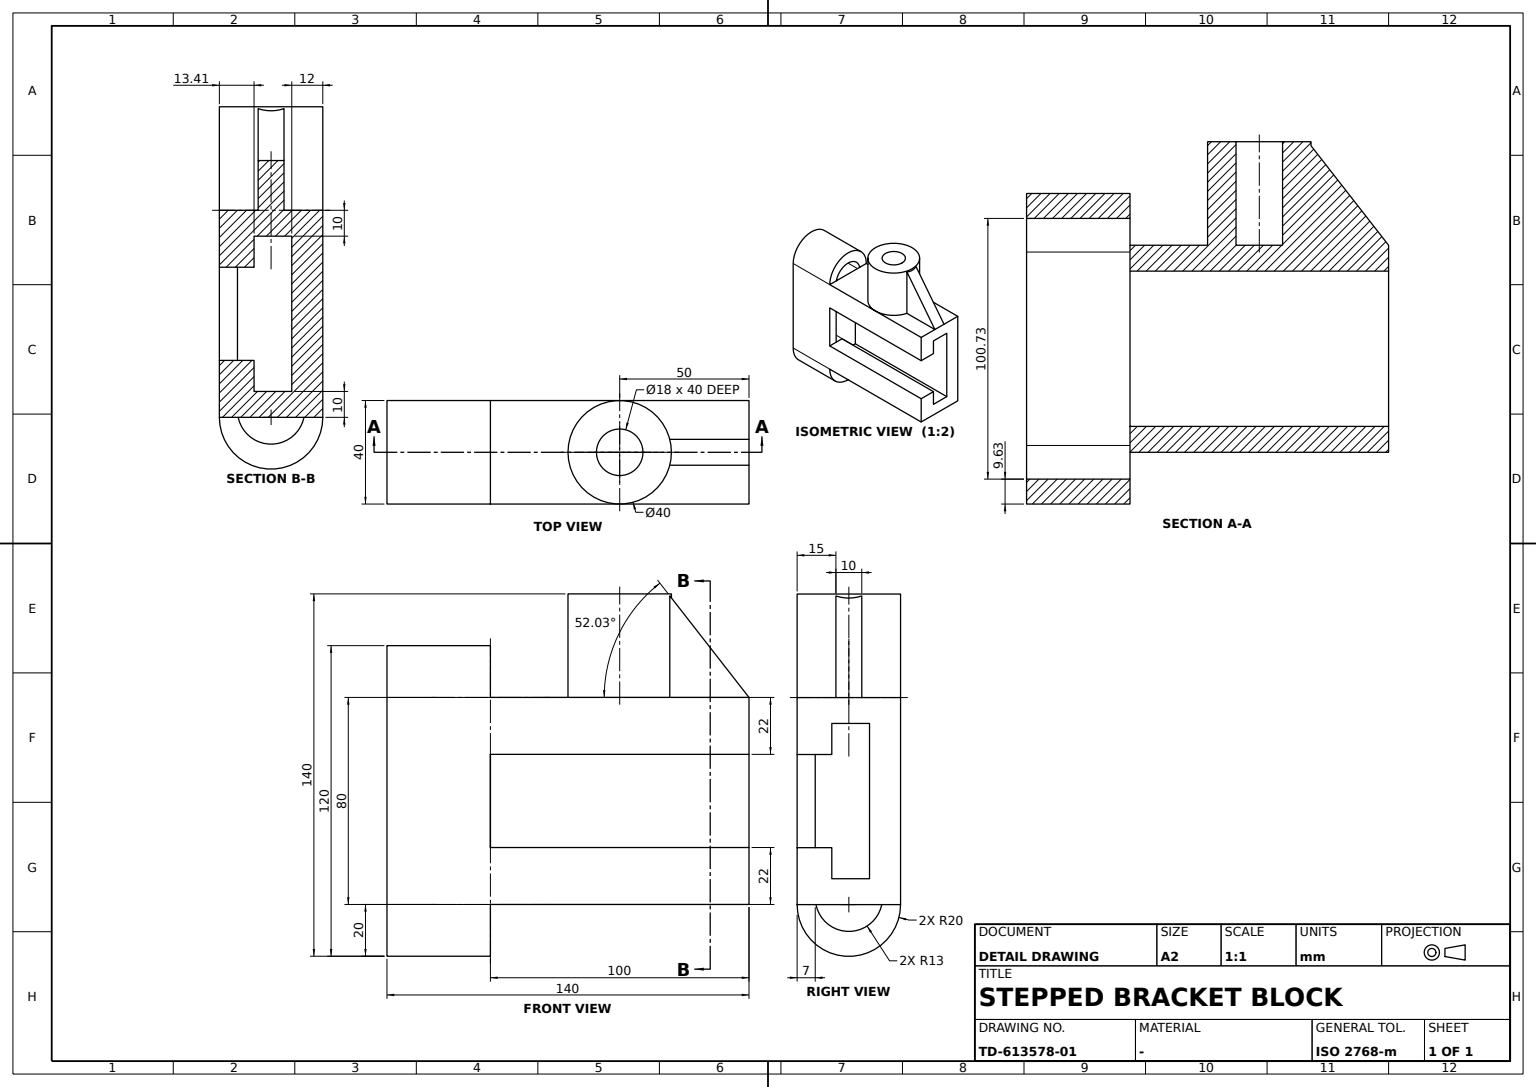
CATIA V5 part; units mm, degrees
sketch "Sketch1" plane through (0, 0, 0) normal (1, 0, 0) x (0, 1, 0)
  point P0 (-20, 40)
  line L0 (-20, 40) -> (20, 40)
  line L1 (20, 40) -> (20, -40)
  point P1 (20, -40)
  line L2 (20, -40) -> (-20, -40)
  point P2 (-20, -40)
  line L3 (-20, -40) -> (-20, -18)
  line L4 (-20, -18) -> (-6.5877, -18)
  line L5 (-6.5877, -18) -> (-6.5877, -30)
  line L6 (-6.5877, -30) -> (8, -30)
  line L7 (8, -30) -> (8, 30)
  line L8 (8, 30) -> (-6.5877, 30)
  point P3 (-6.5877, 30)
  line L9 (-6.5877, 30) -> (-6.5877, 18)
  line L10 (-6.5877, 18) -> (-20, 18)
  point P4 (-20, 18)
  line L11 (-20, 18) -> (-20, 40)
  point P5 (-20, 40)
  dimension "length L2" = 40
  dimension "distance L7 L1" = 12
  dimension "length L1" = 80
  dimension "length L3" = 22
  dimension "length L5" = 12
  dimension "length L11" = 22
  dimension "length L9" = 12
  constraint horizontal L0 x-axis
  constraint horizontal L2 x-axis
  constraint horizontal L4 x-axis
  constraint horizontal L6 x-axis
  constraint horizontal L8 x-axis
  constraint horizontal L10 x-axis
  constraint vertical L1 y-axis
  constraint vertical L3 y-axis
  constraint vertical L5 y-axis
  constraint vertical L7 y-axis
  constraint vertical L9 y-axis
  constraint vertical L11 y-axis
  constraint coincidence P3 L5
  constraint coincidence P4 L3
  constraint coincidence P5 L0
  constraint coincidence P5 P0
  constraint symmetry P2 P1 y-axis
  constraint symmetry L0 L2 x-axis
extrude "Pad1" add sketch "Sketch1" against normal blind 100
sketch "Sketch2" plane through (0, 0, 40) normal (0, 0, 1) x (1, 0, 0)
  circle A0 centre (-50, 0) radius 9
  point P0 (-50, 0)
  circle A1 centre (-50, 0) radius 20
  dimension "distance y axis P0" = 50
  dimension "radius A0" = 9
  dimension "radius A1" = 20
  constraint coincidence P0 x-axis
extrude "Pad2" add sketch "Sketch2" along normal blind 40
ref_plane "Plane1" through (-50, 0, 0) normal (1, 0, 0) x (0, 1, 0)
sketch "Sketch3" plane through (0, 0, 0) normal (0, 1, 0) x (-1, 0, 0)
  point P0 (0, 40)
  line L0 (0, 40) -> (31.2151, 40)
  point P1 (31.2151, 40)
  line L1 (31.2151, 40) -> (31.2151, 80)
  point P2 (31.2151, 80)
  line L2 (31.2151, 80) -> (0, 40)
  line L3 (30, 80) -> (70, 80) construction
  line L4 (0, 40) -> (100, 40) construction
  constraint coincidence P0 y-axis
  constraint coincidence P2 L3
  constraint coincidence P1 L4
  constraint horizontal L0 x-axis
  constraint vertical L1 y-axis
extrude "Pad3" add sketch "Sketch3" along normal mid plane 10
sketch "Sketch4" plane through (-100, 0, 0) normal (-1, 0, 0) x (0, -1, 0)
  line L0 (-20, 40) -> (20, 40)
  line L1 (20, 40) -> (20, -40)
  line L2 (20, -40) -> (-20, -40)
  line L3 (-20, -40) -> (-20, 40)
  line L4 (-20, 40) -> (20, 40) construction
  line L5 (20, 40) -> (20, 18) construction
  line L6 (-20, -40) -> (-20, 40) construction
  line L7 (20, -40) -> (-20, -40) construction
  constraint horizontal L0 x-axis
  constraint horizontal L2 x-axis
  constraint vertical L1 y-axis
  constraint vertical L3 y-axis
  constraint coincidence L4 L0
  constraint coincidence L1 L5
  constraint coincidence L3 L6
  constraint coincidence L2 L7
extrude "Pad4" add sketch "Sketch4" along normal blind 40
ref_plane "Plane2" through (-100, 0, 0) normal (1, 0, 0) x (0, 1, 0)
sketch "Sketch5" plane through (-100, 0, 0) normal (1, 0, 0) x (0, 1, 0)
  circle A0 centre (0, 40) radius 20
  point P0 (0, 40)
  circle A1 centre (0, -40) radius 20
  point P1 (0, -40)
  line L0 (-20, -40) -> (20, -40) construction
  line L1 (5, 40) -> (-5, 40) construction
  dimension "radius A0" = 20
  dimension "radius A1" = 20
  constraint coincidence P0 y-axis
  constraint coincidence P1 y-axis
  constraint coincidence P1 L0
  constraint coincidence P0 L1
extrude "Pad5" add sketch "Sketch5" against normal blind 40
sketch "Sketch6" plane through (-140, 0, 0) normal (-1, 0, 0) x (0, -1, 0)
  line L0 (13, 37.3656) -> (13, -37.3656)
  line L1 (-13, -37.3656) -> (-13, 37.3656)
  point P0 (-13, -37.3656)
  arc A0 (13, 37.3656) -> (-13, 37.3656) centre (0, 37.3656) ccw
  arc A1 (-13, -37.3656) -> (13, -37.3656) centre (0, -37.3656) ccw
  point P1 (-13, -37.3656)
  line L2 (20, 40) -> (20, -40) construction
  dimension "distance L2 L0" = 7
  dimension "radius A1" = 13
  dimension "distance origin A1" = 50.3656
  dimension "distance A0 origin" = 50.3656
  dimension "radius A0" = 13
  constraint vertical L0 y-axis
  constraint vertical L1 y-axis
  constraint symmetry L1 L0 y-axis
  constraint tangency A0 L0
  constraint tangency A1 L1
  constraint coincidence P0 P1
extrude "Pocket1" cut sketch "Sketch6" against normal blind 40
